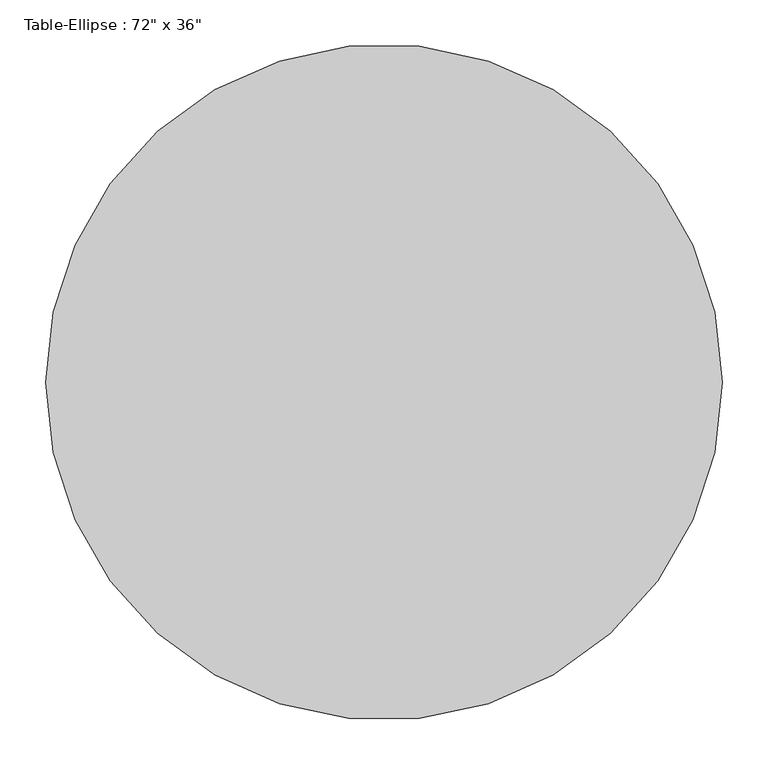
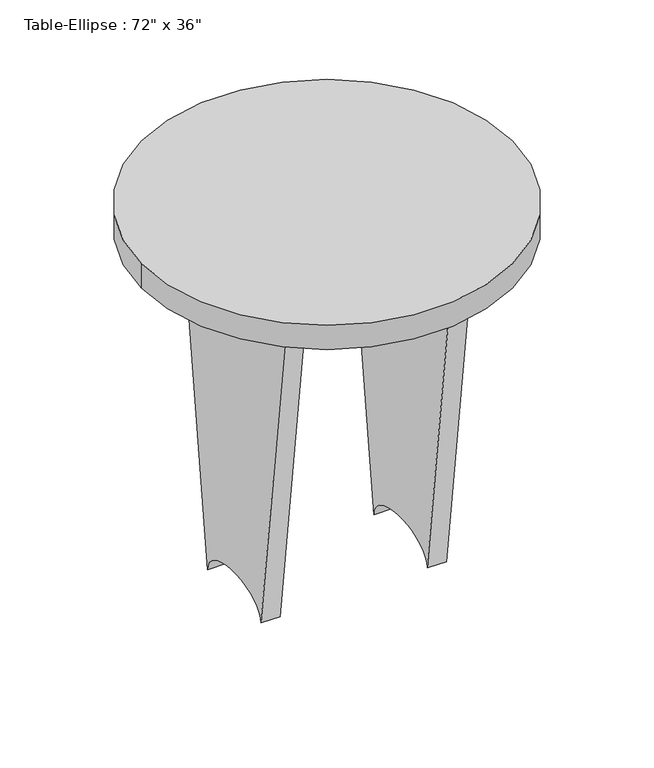
"""IFC4 building model written with IfcOpenShell, lengths in millimetres: furniture geometry."""

from ifc_helpers import new_model, si_unit, point, frame, origin, place, context, project, spatial, circle_curve, ellipse_curve, trimmed, source, transform, mapped, element, save
from ifc_brep_helpers import plane_surface, extruded_surface, advanced_brep


def furniture_b2396e53(model_context):
    return source(origin(), model_context, "Body", "AdvancedBrep", [
        advanced_brep(
        [(-146.05, 19.05, 711.2), (146.05, 19.05, 711.2), (146.05, 19.05, 474.1333333), (-146.05, 19.05, 474.1333333), (-146.05, -19.05, 711.2), (-146.05, -19.05, 474.1333333), (146.05, -19.05, 474.1333333), (146.05, -19.05, 711.2)],
        [
            (0, 1),
            (1, 2),
            (2, 3, ellipse_curve(frame((0.0, 19.05, 474.1333333), z_axis=(0.0, -1.0, 0.0), x_axis=(1.0, 0.0, 0.0)), 146.05, 101.6)),
            (3, 0),
            (4, 5),
            (5, 6, ellipse_curve(frame((0.0, -19.05, 474.1333333), z_axis=(0.0, 1.0, 0.0), x_axis=(1.0, 0.0, 0.0)), 146.05, 101.6)),
            (6, 7),
            (7, 4),
            (0, 4),
            (7, 1),
            (6, 2),
            (5, 3),
        ],
        [
            plane_surface(frame((-146.05, 19.05, 711.2), z_axis=(0.0, 1.0, 0.0), x_axis=(1.0, 0.0, 0.0))),
            plane_surface(frame((-146.05, -19.05, 711.2), z_axis=(0.0, -1.0, 0.0), x_axis=(-1.0, 0.0, 0.0))),
            plane_surface(frame((-146.05, 19.05, 711.2), z_axis=(0.0, 0.0, 1.0), x_axis=(0.0, -1.0, 0.0))),
            plane_surface(frame((146.05, 19.05, 711.2), z_axis=(1.0, 0.0, 0.0), x_axis=(0.0, -1.0, 0.0))),
            extruded_surface(trimmed(ellipse_curve(frame((0.0, -57.15, 474.1333333), z_axis=(0.0, -1.0, 0.0), x_axis=(1.0, 0.0, 0.0)), 146.05, 101.6), [point((146.05, -57.15, 474.1333333))], [point((-146.05, -57.15, 474.1333333))], True, "CARTESIAN"), (0.0, 38.099999999999994, 0.0), 38.099999999999994),
            plane_surface(frame((-146.05, 19.05, 474.1333333), z_axis=(-1.0, 0.0, 0.0), x_axis=(0.0, -1.0, 0.0))),
        ],
        [
            (0, [[1, 2, 3, 4]]),
            (1, [[5, 6, 7, 8]]),
            (2, [[-1, 9, -8, 10]]),
            (3, [[-2, -10, -7, 11]]),
            (4, [[-3, -11, -6, 12]]),
            (5, [[-4, -12, -5, -9]]),
        ],
    ),
        advanced_brep(
        [(184.15, 184.15, 711.2), (184.15, -184.15, 711.2), (184.15, -92.075, 0.0), (184.15, 92.075, 0.0), (146.05, 184.15, 711.2), (146.05, 92.075, 0.0), (146.05, -92.075, 0.0), (146.05, -184.15, 711.2)],
        [
            (0, 1),
            (1, 2),
            (2, 3, ellipse_curve(frame((184.15, 0.0, 0.0), z_axis=(-1.0, 0.0, 0.0), x_axis=(0.0, 1.0, 0.0)), 92.075, 50.8)),
            (3, 0),
            (4, 5),
            (5, 6, ellipse_curve(frame((146.05, 0.0, 0.0), z_axis=(1.0, 0.0, 0.0), x_axis=(0.0, 1.0, 0.0)), 92.075, 50.8)),
            (6, 7),
            (7, 4),
            (0, 4),
            (7, 1),
            (6, 2),
            (5, 3),
        ],
        [
            plane_surface(frame((184.15, -184.15, 711.2), z_axis=(1.0, 0.0, 0.0), x_axis=(0.0, -1.0, 0.0))),
            plane_surface(frame((146.05, -184.15, 711.2), z_axis=(-1.0, 0.0, 0.0), x_axis=(0.0, 1.0, 0.0))),
            plane_surface(frame((184.15, 184.15, 711.2), z_axis=(0.0, 0.0, 1.0), x_axis=(-1.0, 0.0, 0.0))),
            plane_surface(frame((184.15, -184.15, 711.2), z_axis=(0.0, -0.9917233983434902, -0.12839276139268568), x_axis=(-1.0, 0.0, 0.0))),
            extruded_surface(trimmed(ellipse_curve(frame((107.95, 0.0, 0.0), z_axis=(-1.0, 0.0, 0.0), x_axis=(0.0, 1.0, 0.0)), 92.075, 50.8), [point((107.95, -92.075, 0.0))], [point((107.95, 92.075, 0.0))], True, "CARTESIAN"), (38.10000000000001, 0.0, 0.0), 38.10000000000001),
            plane_surface(frame((184.15, 92.075, 0.0), z_axis=(0.0, 0.9917233983434917, -0.12839276139267394), x_axis=(-1.0, 0.0, 0.0))),
        ],
        [
            (0, [[1, 2, 3, 4]]),
            (1, [[5, 6, 7, 8]]),
            (2, [[-1, 9, -8, 10]]),
            (3, [[-2, -10, -7, 11]]),
            (4, [[-3, -11, -6, 12]]),
            (5, [[-4, -12, -5, -9]]),
        ],
    ),
        advanced_brep(
        [(-146.05, 184.15, 711.2), (-146.05, -184.15, 711.2), (-146.05, -92.075, 0.0), (-146.05, 92.075, 0.0), (-184.15, 184.15, 711.2), (-184.15, 92.075, 0.0), (-184.15, -92.075, 0.0), (-184.15, -184.15, 711.2)],
        [
            (0, 1),
            (1, 2),
            (2, 3, ellipse_curve(frame((-146.05, 0.0, 0.0), z_axis=(-1.0, 0.0, 0.0), x_axis=(0.0, 1.0, 0.0)), 92.075, 50.8)),
            (3, 0),
            (4, 5),
            (5, 6, ellipse_curve(frame((-184.15, 0.0, 0.0), z_axis=(1.0, 0.0, 0.0), x_axis=(0.0, 1.0, 0.0)), 92.075, 50.8)),
            (6, 7),
            (7, 4),
            (0, 4),
            (7, 1),
            (6, 2),
            (5, 3),
        ],
        [
            plane_surface(frame((-146.05, -184.15, 711.2), z_axis=(1.0, 0.0, 0.0), x_axis=(0.0, -1.0, 0.0))),
            plane_surface(frame((-184.15, -184.15, 711.2), z_axis=(-1.0, 0.0, 0.0), x_axis=(0.0, 1.0, 0.0))),
            plane_surface(frame((-146.05, 184.15, 711.2), z_axis=(0.0, 0.0, 1.0), x_axis=(-1.0, 0.0, 0.0))),
            plane_surface(frame((-146.05, -184.15, 711.2), z_axis=(0.0, -0.99172339834349, -0.12839276139268746), x_axis=(-1.0, 0.0, 0.0))),
            extruded_surface(trimmed(ellipse_curve(frame((-222.25, 0.0, 0.0), z_axis=(-1.0, 0.0, 0.0), x_axis=(0.0, 1.0, 0.0)), 92.075, 50.8), [point((-222.25, -92.075, 0.0))], [point((-222.25, 92.075, 0.0))], True, "CARTESIAN"), (38.099999999999994, 0.0, 0.0), 38.099999999999994),
            plane_surface(frame((-146.05, 92.075, 0.0), z_axis=(0.0, 0.9917233983434911, -0.12839276139267836), x_axis=(-1.0, 0.0, 0.0))),
        ],
        [
            (0, [[1, 2, 3, 4]]),
            (1, [[5, 6, 7, 8]]),
            (2, [[-1, 9, -8, 10]]),
            (3, [[-2, -10, -7, 11]]),
            (4, [[-3, -11, -6, 12]]),
            (5, [[-4, -12, -5, -9]]),
        ],
    ),
        advanced_brep(
        [(-368.3, 0.0, 762.0), (368.3, 0.0, 762.0), (-368.3, 0.0, 711.2), (368.3, 0.0, 711.2)],
        [
            (0, 1, circle_curve(frame((0.0, 0.0, 762.0), z_axis=(0.0, 0.0, 1.0), x_axis=(1.0, 0.0, 0.0)), 368.3)),
            (1, 0, circle_curve(frame((0.0, 0.0, 762.0), z_axis=(0.0, 0.0, 1.0), x_axis=(1.0, 0.0, 0.0)), 368.3)),
            (2, 3, ellipse_curve(frame((0.0, 0.0, 711.2), z_axis=(0.0, 0.0, -1.0), x_axis=(1.0, 0.0, 0.0)), 368.3, 368.3)),
            (3, 2, ellipse_curve(frame((0.0, 0.0, 711.2), z_axis=(0.0, 0.0, -1.0), x_axis=(1.0, 0.0, 0.0)), 368.3, 368.3)),
            (0, 2),
            (3, 1),
        ],
        [
            plane_surface(frame((368.3, 0.0, 762.0), z_axis=(0.0, 0.0, 1.0), x_axis=(0.0, 1.0, 0.0))),
            plane_surface(frame((368.3, 0.0, 711.2), z_axis=(0.0, 0.0, -1.0), x_axis=(0.0, -1.0, 0.0))),
            extruded_surface(trimmed(ellipse_curve(frame((0.0, 0.0, 660.4), z_axis=(0.0, 0.0, 1.0), x_axis=(1.0, 0.0, 0.0)), 368.3, 368.3), [point((-368.3, 0.0, 660.4))], [point((368.3, 0.0, 660.4))], True, "CARTESIAN"), (0.0, 0.0, 50.80000000000007), 50.80000000000007),
            extruded_surface(trimmed(ellipse_curve(frame((0.0, 0.0, 660.4), z_axis=(0.0, 0.0, 1.0), x_axis=(1.0, 0.0, 0.0)), 368.3, 368.3), [point((368.3, 0.0, 660.4))], [point((-368.3, 0.0, 660.4))], True, "CARTESIAN"), (0.0, 0.0, 50.80000000000007), 50.80000000000007),
        ],
        [
            (0, [[1, 2]]),
            (1, [[3, 4]]),
            (2, [[-1, 5, -4, 6]]),
            (3, [[-2, -6, -3, -5]]),
        ],
    ),
    ])


if __name__ == "__main__":
    model = new_model("IFC4")
    model_context = context("Model", 3, world=origin())
    ifc_project = project(units=[si_unit("LENGTHUNIT", "METRE", prefix="MILLI")], contexts=[model_context])
    site = spatial("IfcSite", under=ifc_project)
    building = spatial("IfcBuilding", under=site)
    placement = place(None, origin())
    furniture_shape = furniture_b2396e53(model_context)
    element("IfcFurniture", 1, ObjectType="Table-Ellipse : 72\" x 36\"", at=placement, inside=building, context=model_context, shape_type="MappedRepresentation", body=[
        mapped(furniture_shape, transform((0.0, 0.0, 0.0), x_axis=(1.0, 0.0, 0.0), y_axis=(0.0, 1.0, 0.0), z_axis=(0.0, 0.0, 1.0))),
    ])
    save(model, "model.ifc")

# Revit data of these elements
# Type "Table-Ellipse : 72\" x 36\""
#   Assembly Code = "E2020200"
#   Half Width = 1' - 2 1/2"
#   Half Length = 1' - 2 1/2"
#   Height = 2' - 6"
#   Length = 2' - 5"
#   Width = 2' - 5"
#   Base Material = Birch
#   Top Material = Laminate - Black
#   Default Elevation = 0
# Element 1 (IfcFurniture, "Table-Ellipse : 72\" x 36\"")
#   Materials on its faces: "Birch", "Laminate - Black"
# Materials
#   "Birch": class "Wood", colour RGB 224 178 126, transparency 0, Description = "Betula Alleghaniensis", Cost = 0
#   "Laminate - Black": colour RGB 0 0 0, transparency 0
